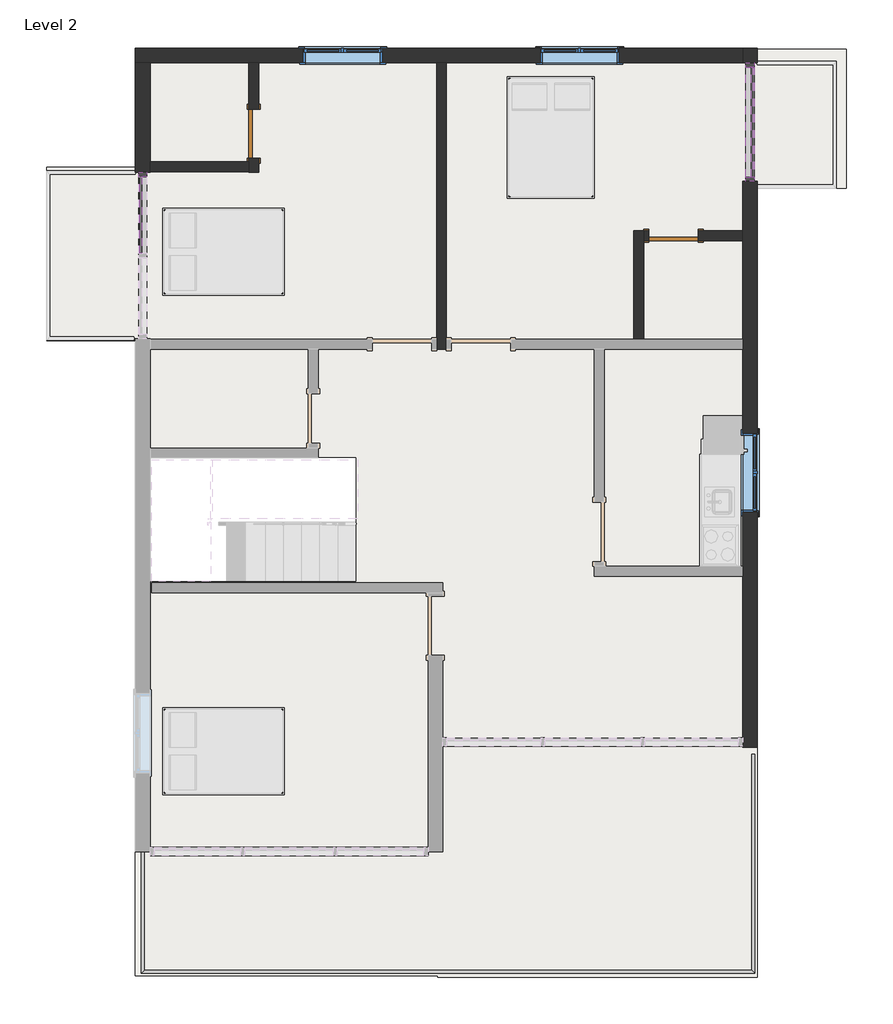
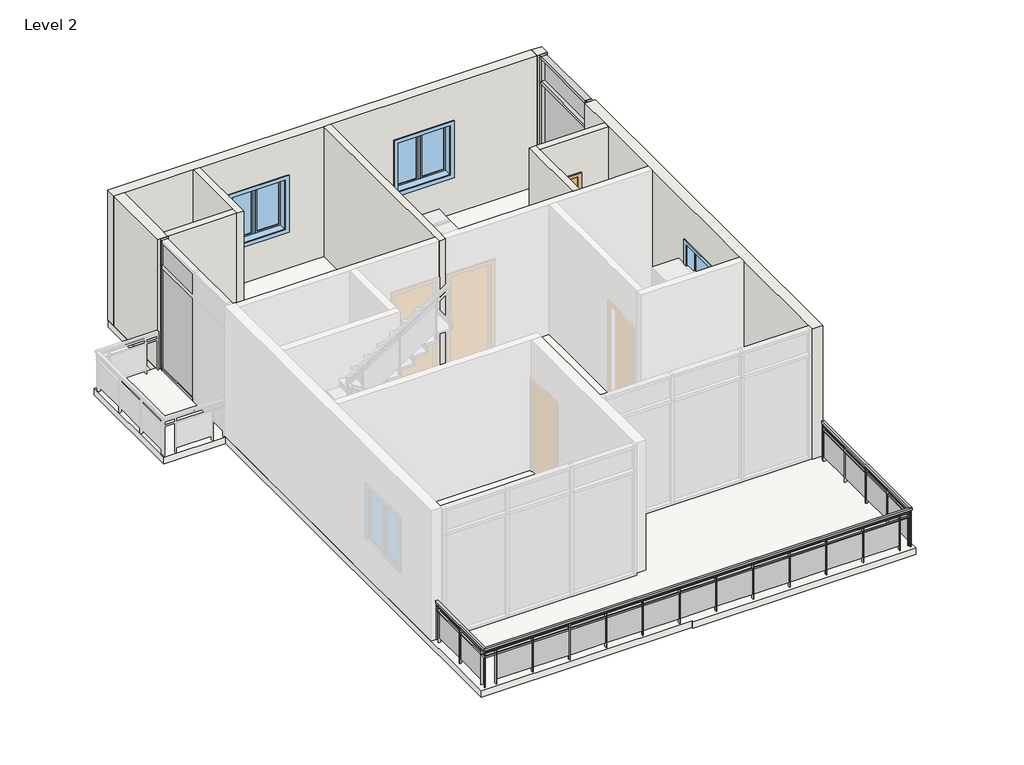
# One storey, part 2 of 3: 10 members, 9 walls, 4 plates, 3 windows, 2 doors, 1 railing, 1 slab.
"""IFC4 building model written with IfcOpenShell, lengths in millimetres."""

from ifc_helpers import new_model, si_unit, frame, origin, place, context, project, spatial, polyline, outline, extrude, faceted_brep, transform, mapped, element, save
from components import single_flush_2_5_e2b13fe9, single_flush_2_5_a9addea7, member_ee409385, member_47bfaf8a, member_43f7a5f1, member_7bc42366, member_cba59155, system_panel_glazed_153bb9bb, system_panel_glazed_f2c52b8f, system_panel_glazed_2d78c1f3, system_panel_glazed_c29578c4, window_8af0dca1

model = new_model("IFC4")

# Units and contexts
model_context = context("Model", 3, world=origin())
ifc_project = project(units=[si_unit("LENGTHUNIT", "METRE", prefix="MILLI")], contexts=[model_context])

# Site, building, storey
site = spatial("IfcSite", under=ifc_project)
building = spatial("IfcBuilding", under=site)
storey = spatial("IfcBuildingStorey", under=building, Name="Level 2", Elevation=3200.4)

# Doors
placement = place(None, origin())
single_flush_2_5_shape = single_flush_2_5_e2b13fe9(model_context)
element("IfcDoor", 1, ObjectType="Single-Flush : 2.5'", at=placement, inside=storey, context=model_context, shape_type="MappedRepresentation", body=[
    mapped(single_flush_2_5_shape, transform((-5884.6647018, 6365.0825188, 3200.4), x_axis=(0.0, -1.0, 0.0), y_axis=(1.0, 0.0, 0.0), z_axis=(0.0, 0.0, 1.0))),
])
single_flush_2_5_2_shape = single_flush_2_5_a9addea7(model_context)
element("IfcDoor", 2, ObjectType="Single-Flush : 2.5'", at=placement, inside=storey, context=model_context, shape_type="MappedRepresentation", body=[
    mapped(single_flush_2_5_2_shape, transform((592.3352982, 4790.2825188, 3200.4), x_axis=(-1.0, 0.0, 0.0), y_axis=(0.0, -1.0, 0.0), z_axis=(0.0, 0.0, 1.0))),
])

# Members
member_shape = member_ee409385(model_context)
element("IfcMember", 3, ObjectType="Rectangular Mullion : 2.5\" x 5\" rectangular", at=placement, inside=storey, context=model_context, shape_type="MappedRepresentation", body=[
    mapped(member_shape, transform((1773.4352982, 5628.4825188, 3200.4), x_axis=(0.0, -1.0, 0.0), y_axis=(-1.0, 0.0, 0.0), z_axis=(0.0, 0.0, -1.0))),
])
element("IfcMember", 4, ObjectType="Rectangular Mullion : 2.5\" x 5\" rectangular", at=placement, inside=storey, context=model_context, shape_type="MappedRepresentation", body=[
    mapped(member_shape, transform((1773.4352982, 7457.2825188, 5638.8), x_axis=(0.0, 1.0, 0.0), y_axis=(-1.0, 0.0, 0.0), z_axis=(0.0, 0.0, 1.0))),
])
member_2_shape = member_47bfaf8a(model_context)
element("IfcMember", 5, ObjectType="Rectangular Mullion : 2.5\" x 5\" rectangular", at=placement, inside=storey, context=model_context, shape_type="MappedRepresentation", body=[
    mapped(member_2_shape, transform((1773.4352982, 5628.4825188, 5638.8), x_axis=(0.0, -1.0, 0.0), y_axis=(-1.0, 0.0, 0.0), z_axis=(0.0, 0.0, -1.0))),
])
element("IfcMember", 6, ObjectType="Rectangular Mullion : 2.5\" x 5\" rectangular", at=placement, inside=storey, context=model_context, shape_type="MappedRepresentation", body=[
    mapped(member_2_shape, transform((1773.4352982, 7457.2825188, 6248.4), x_axis=(0.0, 1.0, 0.0), y_axis=(-1.0, 0.0, 0.0), z_axis=(0.0, 0.0, 1.0))),
])
member_3_shape = member_43f7a5f1(model_context)
element("IfcMember", 7, ObjectType="Rectangular Mullion : 2.5\" x 5\" rectangular", at=placement, inside=storey, context=model_context, shape_type="MappedRepresentation", body=[
    mapped(member_3_shape, transform((-7599.1647018, 5704.6825188, 3200.4), x_axis=(0.0, 0.0, -1.0), y_axis=(-1.0, 0.0, 0.0), z_axis=(0.0, 1.0, 0.0))),
])
element("IfcMember", 8, ObjectType="Rectangular Mullion : 2.5\" x 5\" rectangular", at=placement, inside=storey, context=model_context, shape_type="MappedRepresentation", body=[
    mapped(member_shape, transform((-7599.1647018, 5768.1825188, 5638.8), x_axis=(0.0, 1.0, 0.0), y_axis=(-1.0, 0.0, 0.0), z_axis=(0.0, 0.0, 1.0))),
])
element("IfcMember", 9, ObjectType="Rectangular Mullion : 2.5\" x 5\" rectangular", at=placement, inside=storey, context=model_context, shape_type="MappedRepresentation", body=[
    mapped(member_2_shape, transform((-7599.1647018, 5768.1825188, 6248.4), x_axis=(0.0, 1.0, 0.0), y_axis=(-1.0, 0.0, 0.0), z_axis=(0.0, 0.0, 1.0))),
])
member_4_shape = member_7bc42366(model_context)
element("IfcMember", 10, ObjectType="Rectangular Mullion : 2.5\" x 5\" rectangular", at=placement, inside=storey, context=model_context, shape_type="MappedRepresentation", body=[
    mapped(member_4_shape, transform((1773.4352982, 5691.9825188, 6248.4), x_axis=(0.0, 0.0, 1.0), y_axis=(-1.0, 0.0, 0.0), z_axis=(0.0, -1.0, 0.0))),
])
element("IfcMember", 11, ObjectType="Rectangular Mullion : 2.5\" x 5\" rectangular", at=placement, inside=storey, context=model_context, shape_type="MappedRepresentation", body=[
    mapped(member_4_shape, transform((1773.4352982, 7393.7825188, 3200.4), x_axis=(0.0, 0.0, -1.0), y_axis=(-1.0, 0.0, 0.0), z_axis=(0.0, 1.0, 0.0))),
])
member_5_shape = member_cba59155(model_context)
element("IfcMember", 12, ObjectType="Rectangular Mullion : 2.5\" x 5\" rectangular", at=placement, inside=storey, context=model_context, shape_type="MappedRepresentation", body=[
    mapped(member_5_shape, transform((1773.4352982, 5691.9825188, 5638.8), x_axis=(0.0, 0.0, 1.0), y_axis=(-1.0, 0.0, 0.0), z_axis=(0.0, -1.0, 0.0))),
])

# Plates
system_panel_glazed_shape = system_panel_glazed_153bb9bb(model_context)
element("IfcPlate", 13, ObjectType="System Panel : Glazed", at=placement, inside=storey, context=model_context, shape_type="MappedRepresentation", body=[
    mapped(system_panel_glazed_shape, transform((-7599.1647018, 5110.9575188, 3263.9), x_axis=(0.0, -1.0, 0.0), y_axis=(1.0, 0.0, 0.0), z_axis=(0.0, 0.0, 1.0))),
])
system_panel_glazed_2_shape = system_panel_glazed_f2c52b8f(model_context)
element("IfcPlate", 14, ObjectType="System Panel : Glazed", at=placement, inside=storey, context=model_context, shape_type="MappedRepresentation", body=[
    mapped(system_panel_glazed_2_shape, transform((-7599.1647018, 5110.9575188, 5670.55), x_axis=(0.0, -1.0, 0.0), y_axis=(1.0, 0.0, 0.0), z_axis=(0.0, 0.0, 1.0))),
])
system_panel_glazed_3_shape = system_panel_glazed_2d78c1f3(model_context)
element("IfcPlate", 15, ObjectType="System Panel : Glazed", at=placement, inside=storey, context=model_context, shape_type="MappedRepresentation", body=[
    mapped(system_panel_glazed_3_shape, transform((1773.4352982, 6542.8825188, 3263.9), x_axis=(0.0, -1.0, 0.0), y_axis=(1.0, 0.0, 0.0), z_axis=(0.0, 0.0, 1.0))),
])
system_panel_glazed_4_shape = system_panel_glazed_c29578c4(model_context)
element("IfcPlate", 16, ObjectType="System Panel : Glazed", at=placement, inside=storey, context=model_context, shape_type="MappedRepresentation", body=[
    mapped(system_panel_glazed_4_shape, transform((1773.4352982, 6542.8825188, 5670.55), x_axis=(0.0, -1.0, 0.0), y_axis=(1.0, 0.0, 0.0), z_axis=(0.0, 0.0, 1.0))),
])

# Railing
element("IfcRailing", 17, ObjectType="Glass Panel - Bottom Fill", at=placement, inside=storey, context=model_context, shape_type="SolidModel", body=[
    faceted_brep([(-7573.7647018, -4715.6674812, 4114.8), (-7573.7647018, -4715.6674812, 4064.0), (-7624.5647018, -4715.6674812, 4064.0), (-7624.5647018, -4715.6674812, 4114.8), (-7573.7647018, -6544.4674812, 4114.8), (-7573.7647018, -6544.4674812, 4064.0), (-7624.5647018, -6595.2674812, 4064.0), (-7624.5647018, -6595.2674812, 4114.8), (1798.8352982, -6544.4674812, 4114.8), (1798.8352982, -6544.4674812, 4064.0), (1849.6352982, -6595.2674812, 4064.0), (1849.6352982, -6595.2674812, 4114.8), (1798.8352982, -3217.0674812, 4114.8), (1849.6352982, -3217.0674812, 4114.8), (1849.6352982, -3217.0674812, 4064.0), (1798.8352982, -3217.0674812, 4064.0)], [[[0, 1, 2, 3]], [[1, 0, 4, 5]], [[2, 1, 5, 6]], [[3, 2, 6, 7]], [[0, 3, 7, 4]], [[5, 4, 8, 9]], [[6, 5, 9, 10]], [[7, 6, 10, 11]], [[4, 7, 11, 8]], [[12, 13, 14, 15]], [[9, 8, 12, 15]], [[10, 9, 15, 14]], [[11, 10, 14, 13]], [[8, 11, 13, 12]]]),
    faceted_brep([(-7611.8647018, -4715.6674812, 4025.9), (-7586.4647018, -4715.6674812, 4025.9), (-7586.4647018, -4715.6674812, 4000.5), (-7611.8647018, -4715.6674812, 4000.5), (-7611.8647018, -6582.5674812, 4025.9), (-7586.4647018, -6557.1674812, 4025.9), (-7586.4647018, -6557.1674812, 4000.5), (-7611.8647018, -6582.5674812, 4000.5), (1836.9352982, -6582.5674812, 4025.9), (1811.5352982, -6557.1674812, 4025.9), (1811.5352982, -6557.1674812, 4000.5), (1836.9352982, -6582.5674812, 4000.5), (1836.9352982, -3217.0674812, 4025.9), (1836.9352982, -3217.0674812, 4000.5), (1811.5352982, -3217.0674812, 4000.5), (1811.5352982, -3217.0674812, 4025.9)], [[[0, 1, 2, 3]], [[1, 0, 4, 5]], [[2, 1, 5, 6]], [[3, 2, 6, 7]], [[0, 3, 7, 4]], [[5, 4, 8, 9]], [[6, 5, 9, 10]], [[7, 6, 10, 11]], [[4, 7, 11, 8]], [[12, 13, 14, 15]], [[9, 8, 12, 15]], [[10, 9, 15, 14]], [[11, 10, 14, 13]], [[8, 11, 13, 12]]]),
    faceted_brep([(-7611.8647018, -4715.6674812, 3924.3), (-7586.4647018, -4715.6674812, 3924.3), (-7586.4647018, -4715.6674812, 3898.9), (-7611.8647018, -4715.6674812, 3898.9), (-7611.8647018, -6582.5674812, 3924.3), (-7586.4647018, -6557.1674812, 3924.3), (-7586.4647018, -6557.1674812, 3898.9), (-7611.8647018, -6582.5674812, 3898.9), (1836.9352982, -6582.5674812, 3924.3), (1811.5352982, -6557.1674812, 3924.3), (1811.5352982, -6557.1674812, 3898.9), (1836.9352982, -6582.5674812, 3898.9), (1836.9352982, -3217.0674812, 3924.3), (1836.9352982, -3217.0674812, 3898.9), (1811.5352982, -3217.0674812, 3898.9), (1811.5352982, -3217.0674812, 3924.3)], [[[0, 1, 2, 3]], [[1, 0, 4, 5]], [[2, 1, 5, 6]], [[3, 2, 6, 7]], [[0, 3, 7, 4]], [[5, 4, 8, 9]], [[6, 5, 9, 10]], [[7, 6, 10, 11]], [[4, 7, 11, 8]], [[12, 13, 14, 15]], [[9, 8, 12, 15]], [[10, 9, 15, 14]], [[11, 10, 14, 13]], [[8, 11, 13, 12]]]),
    extrude(outline(polyline([(1849.6352982, -3274.2174812), (1798.8352982, -3274.2174812), (1798.8352982, -3261.5174812), (1849.6352982, -3261.5174812), (1849.6352982, -3274.2174812)])), frame((0.0, 0.0, 3200.4), z_axis=(0.0, 0.0, 1.0), x_axis=(1.0, 0.0, 0.0)), (0.0, 0.0, 1.0), 863.6),
    extrude(outline(polyline([(1817.7001412, -4080.6674812), (1817.7001412, -3267.8674812), (1824.0501412, -3267.8674812), (1824.0501412, -4080.6674812), (1817.7001412, -4080.6674812)])), frame((0.0, 0.0, 3302.0), z_axis=(0.0, 0.0, 1.0), x_axis=(1.0, 0.0, 0.0)), (0.0, 0.0, 1.0), 596.9),
    extrude(outline(polyline([(1849.6352982, -4087.0174812), (1798.8352982, -4087.0174812), (1798.8352982, -4074.3174812), (1849.6352982, -4074.3174812), (1849.6352982, -4087.0174812)])), frame((0.0, 0.0, 3200.4), z_axis=(0.0, 0.0, 1.0), x_axis=(1.0, 0.0, 0.0)), (0.0, 0.0, 1.0), 863.6),
    extrude(outline(polyline([(1817.7001412, -4893.4674812), (1817.7001412, -4080.6674812), (1824.0501412, -4080.6674812), (1824.0501412, -4893.4674812), (1817.7001412, -4893.4674812)])), frame((0.0, 0.0, 3302.0), z_axis=(0.0, 0.0, 1.0), x_axis=(1.0, 0.0, 0.0)), (0.0, 0.0, 1.0), 596.9),
    extrude(outline(polyline([(1849.6352982, -4899.8174812), (1798.8352982, -4899.8174812), (1798.8352982, -4887.1174812), (1849.6352982, -4887.1174812), (1849.6352982, -4899.8174812)])), frame((0.0, 0.0, 3200.4), z_axis=(0.0, 0.0, 1.0), x_axis=(1.0, 0.0, 0.0)), (0.0, 0.0, 1.0), 863.6),
    extrude(outline(polyline([(1817.7001412, -5706.2674812), (1817.7001412, -4893.4674812), (1824.0501412, -4893.4674812), (1824.0501412, -5706.2674812), (1817.7001412, -5706.2674812)])), frame((0.0, 0.0, 3302.0), z_axis=(0.0, 0.0, 1.0), x_axis=(1.0, 0.0, 0.0)), (0.0, 0.0, 1.0), 596.9),
    extrude(outline(polyline([(1849.6352982, -5712.6174812), (1798.8352982, -5712.6174812), (1798.8352982, -5699.9174812), (1849.6352982, -5699.9174812), (1849.6352982, -5712.6174812)])), frame((0.0, 0.0, 3200.4), z_axis=(0.0, 0.0, 1.0), x_axis=(1.0, 0.0, 0.0)), (0.0, 0.0, 1.0), 863.6),
    extrude(outline(polyline([(1817.7001412, -6519.0674812), (1817.7001412, -5706.2674812), (1824.0501412, -5706.2674812), (1824.0501412, -6519.0674812), (1817.7001412, -6519.0674812)])), frame((0.0, 0.0, 3302.0), z_axis=(0.0, 0.0, 1.0), x_axis=(1.0, 0.0, 0.0)), (0.0, 0.0, 1.0), 596.9),
    extrude(outline(polyline([(1849.6352982, -6525.4174812), (1798.8352982, -6525.4174812), (1798.8352982, -6512.7174812), (1849.6352982, -6512.7174812), (1849.6352982, -6525.4174812)])), frame((0.0, 0.0, 3200.4), z_axis=(0.0, 0.0, 1.0), x_axis=(1.0, 0.0, 0.0)), (0.0, 0.0, 1.0), 863.6),
    extrude(outline(polyline([(1576.5852982, -6595.2674812), (1576.5852982, -6544.4674812), (1589.2852982, -6544.4674812), (1589.2852982, -6595.2674812), (1576.5852982, -6595.2674812)])), frame((0.0, 0.0, 3200.4), z_axis=(0.0, 0.0, 1.0), x_axis=(1.0, 0.0, 0.0)), (0.0, 0.0, 1.0), 863.6),
    extrude(outline(polyline([(770.1352982, -6563.3323242), (1582.9352982, -6563.3323242), (1582.9352982, -6569.6823242), (770.1352982, -6569.6823242), (770.1352982, -6563.3323242)])), frame((0.0, 0.0, 3302.0), z_axis=(0.0, 0.0, 1.0), x_axis=(1.0, 0.0, 0.0)), (0.0, 0.0, 1.0), 596.9),
    extrude(outline(polyline([(763.7852982, -6595.2674812), (763.7852982, -6544.4674812), (776.4852982, -6544.4674812), (776.4852982, -6595.2674812), (763.7852982, -6595.2674812)])), frame((0.0, 0.0, 3200.4), z_axis=(0.0, 0.0, 1.0), x_axis=(1.0, 0.0, 0.0)), (0.0, 0.0, 1.0), 863.6),
    extrude(outline(polyline([(-42.6647018, -6563.3323242), (770.1352982, -6563.3323242), (770.1352982, -6569.6823242), (-42.6647018, -6569.6823242), (-42.6647018, -6563.3323242)])), frame((0.0, 0.0, 3302.0), z_axis=(0.0, 0.0, 1.0), x_axis=(1.0, 0.0, 0.0)), (0.0, 0.0, 1.0), 596.9),
    extrude(outline(polyline([(-49.0147018, -6595.2674812), (-49.0147018, -6544.4674812), (-36.3147018, -6544.4674812), (-36.3147018, -6595.2674812), (-49.0147018, -6595.2674812)])), frame((0.0, 0.0, 3200.4), z_axis=(0.0, 0.0, 1.0), x_axis=(1.0, 0.0, 0.0)), (0.0, 0.0, 1.0), 863.6),
    extrude(outline(polyline([(-855.4647018, -6563.3323242), (-42.6647018, -6563.3323242), (-42.6647018, -6569.6823242), (-855.4647018, -6569.6823242), (-855.4647018, -6563.3323242)])), frame((0.0, 0.0, 3302.0), z_axis=(0.0, 0.0, 1.0), x_axis=(1.0, 0.0, 0.0)), (0.0, 0.0, 1.0), 596.9),
    extrude(outline(polyline([(-861.8147018, -6595.2674812), (-861.8147018, -6544.4674812), (-849.1147018, -6544.4674812), (-849.1147018, -6595.2674812), (-861.8147018, -6595.2674812)])), frame((0.0, 0.0, 3200.4), z_axis=(0.0, 0.0, 1.0), x_axis=(1.0, 0.0, 0.0)), (0.0, 0.0, 1.0), 863.6),
    extrude(outline(polyline([(-1668.2647018, -6563.3323242), (-855.4647018, -6563.3323242), (-855.4647018, -6569.6823242), (-1668.2647018, -6569.6823242), (-1668.2647018, -6563.3323242)])), frame((0.0, 0.0, 3302.0), z_axis=(0.0, 0.0, 1.0), x_axis=(1.0, 0.0, 0.0)), (0.0, 0.0, 1.0), 596.9),
    extrude(outline(polyline([(-1674.6147018, -6595.2674812), (-1674.6147018, -6544.4674812), (-1661.9147018, -6544.4674812), (-1661.9147018, -6595.2674812), (-1674.6147018, -6595.2674812)])), frame((0.0, 0.0, 3200.4), z_axis=(0.0, 0.0, 1.0), x_axis=(1.0, 0.0, 0.0)), (0.0, 0.0, 1.0), 863.6),
    extrude(outline(polyline([(-2481.0647018, -6563.3323242), (-1668.2647018, -6563.3323242), (-1668.2647018, -6569.6823242), (-2481.0647018, -6569.6823242), (-2481.0647018, -6563.3323242)])), frame((0.0, 0.0, 3302.0), z_axis=(0.0, 0.0, 1.0), x_axis=(1.0, 0.0, 0.0)), (0.0, 0.0, 1.0), 596.9),
    extrude(outline(polyline([(-2487.4147018, -6595.2674812), (-2487.4147018, -6544.4674812), (-2474.7147018, -6544.4674812), (-2474.7147018, -6595.2674812), (-2487.4147018, -6595.2674812)])), frame((0.0, 0.0, 3200.4), z_axis=(0.0, 0.0, 1.0), x_axis=(1.0, 0.0, 0.0)), (0.0, 0.0, 1.0), 863.6),
    extrude(outline(polyline([(-3293.8647018, -6563.3323242), (-2481.0647018, -6563.3323242), (-2481.0647018, -6569.6823242), (-3293.8647018, -6569.6823242), (-3293.8647018, -6563.3323242)])), frame((0.0, 0.0, 3302.0), z_axis=(0.0, 0.0, 1.0), x_axis=(1.0, 0.0, 0.0)), (0.0, 0.0, 1.0), 596.9),
    extrude(outline(polyline([(-3300.2147018, -6595.2674812), (-3300.2147018, -6544.4674812), (-3287.5147018, -6544.4674812), (-3287.5147018, -6595.2674812), (-3300.2147018, -6595.2674812)])), frame((0.0, 0.0, 3200.4), z_axis=(0.0, 0.0, 1.0), x_axis=(1.0, 0.0, 0.0)), (0.0, 0.0, 1.0), 863.6),
    extrude(outline(polyline([(-4106.6647018, -6563.3323242), (-3293.8647018, -6563.3323242), (-3293.8647018, -6569.6823242), (-4106.6647018, -6569.6823242), (-4106.6647018, -6563.3323242)])), frame((0.0, 0.0, 3302.0), z_axis=(0.0, 0.0, 1.0), x_axis=(1.0, 0.0, 0.0)), (0.0, 0.0, 1.0), 596.9),
    extrude(outline(polyline([(-4113.0147018, -6595.2674812), (-4113.0147018, -6544.4674812), (-4100.3147018, -6544.4674812), (-4100.3147018, -6595.2674812), (-4113.0147018, -6595.2674812)])), frame((0.0, 0.0, 3200.4), z_axis=(0.0, 0.0, 1.0), x_axis=(1.0, 0.0, 0.0)), (0.0, 0.0, 1.0), 863.6),
    extrude(outline(polyline([(-4919.4647018, -6563.3323242), (-4106.6647018, -6563.3323242), (-4106.6647018, -6569.6823242), (-4919.4647018, -6569.6823242), (-4919.4647018, -6563.3323242)])), frame((0.0, 0.0, 3302.0), z_axis=(0.0, 0.0, 1.0), x_axis=(1.0, 0.0, 0.0)), (0.0, 0.0, 1.0), 596.9),
    extrude(outline(polyline([(-4925.8147018, -6595.2674812), (-4925.8147018, -6544.4674812), (-4913.1147018, -6544.4674812), (-4913.1147018, -6595.2674812), (-4925.8147018, -6595.2674812)])), frame((0.0, 0.0, 3200.4), z_axis=(0.0, 0.0, 1.0), x_axis=(1.0, 0.0, 0.0)), (0.0, 0.0, 1.0), 863.6),
    extrude(outline(polyline([(-5732.2647018, -6563.3323242), (-4919.4647018, -6563.3323242), (-4919.4647018, -6569.6823242), (-5732.2647018, -6569.6823242), (-5732.2647018, -6563.3323242)])), frame((0.0, 0.0, 3302.0), z_axis=(0.0, 0.0, 1.0), x_axis=(1.0, 0.0, 0.0)), (0.0, 0.0, 1.0), 596.9),
    extrude(outline(polyline([(-5738.6147018, -6595.2674812), (-5738.6147018, -6544.4674812), (-5725.9147018, -6544.4674812), (-5725.9147018, -6595.2674812), (-5738.6147018, -6595.2674812)])), frame((0.0, 0.0, 3200.4), z_axis=(0.0, 0.0, 1.0), x_axis=(1.0, 0.0, 0.0)), (0.0, 0.0, 1.0), 863.6),
    extrude(outline(polyline([(-6545.0647018, -6563.3323242), (-5732.2647018, -6563.3323242), (-5732.2647018, -6569.6823242), (-6545.0647018, -6569.6823242), (-6545.0647018, -6563.3323242)])), frame((0.0, 0.0, 3302.0), z_axis=(0.0, 0.0, 1.0), x_axis=(1.0, 0.0, 0.0)), (0.0, 0.0, 1.0), 596.9),
    extrude(outline(polyline([(-6551.4147018, -6595.2674812), (-6551.4147018, -6544.4674812), (-6538.7147018, -6544.4674812), (-6538.7147018, -6595.2674812), (-6551.4147018, -6595.2674812)])), frame((0.0, 0.0, 3200.4), z_axis=(0.0, 0.0, 1.0), x_axis=(1.0, 0.0, 0.0)), (0.0, 0.0, 1.0), 863.6),
    extrude(outline(polyline([(-7357.8647018, -6563.3323242), (-6545.0647018, -6563.3323242), (-6545.0647018, -6569.6823242), (-7357.8647018, -6569.6823242), (-7357.8647018, -6563.3323242)])), frame((0.0, 0.0, 3302.0), z_axis=(0.0, 0.0, 1.0), x_axis=(1.0, 0.0, 0.0)), (0.0, 0.0, 1.0), 596.9),
    extrude(outline(polyline([(-7364.2147018, -6595.2674812), (-7364.2147018, -6544.4674812), (-7351.5147018, -6544.4674812), (-7351.5147018, -6595.2674812), (-7364.2147018, -6595.2674812)])), frame((0.0, 0.0, 3200.4), z_axis=(0.0, 0.0, 1.0), x_axis=(1.0, 0.0, 0.0)), (0.0, 0.0, 1.0), 863.6),
    extrude(outline(polyline([(-7624.5647018, -6449.2174812), (-7573.7647018, -6449.2174812), (-7573.7647018, -6461.9174812), (-7624.5647018, -6461.9174812), (-7624.5647018, -6449.2174812)])), frame((0.0, 0.0, 3200.4), z_axis=(0.0, 0.0, 1.0), x_axis=(1.0, 0.0, 0.0)), (0.0, 0.0, 1.0), 863.6),
    extrude(outline(polyline([(-7592.6295448, -5642.7674812), (-7592.6295448, -6455.5674812), (-7598.9795448, -6455.5674812), (-7598.9795448, -5642.7674812), (-7592.6295448, -5642.7674812)])), frame((0.0, 0.0, 3302.0), z_axis=(0.0, 0.0, 1.0), x_axis=(1.0, 0.0, 0.0)), (0.0, 0.0, 1.0), 596.9),
    extrude(outline(polyline([(-7624.5647018, -5636.4174812), (-7573.7647018, -5636.4174812), (-7573.7647018, -5649.1174812), (-7624.5647018, -5649.1174812), (-7624.5647018, -5636.4174812)])), frame((0.0, 0.0, 3200.4), z_axis=(0.0, 0.0, 1.0), x_axis=(1.0, 0.0, 0.0)), (0.0, 0.0, 1.0), 863.6),
    extrude(outline(polyline([(-7592.6295448, -4829.9674812), (-7592.6295448, -5642.7674812), (-7598.9795448, -5642.7674812), (-7598.9795448, -4829.9674812), (-7592.6295448, -4829.9674812)])), frame((0.0, 0.0, 3302.0), z_axis=(0.0, 0.0, 1.0), x_axis=(1.0, 0.0, 0.0)), (0.0, 0.0, 1.0), 596.9),
    extrude(outline(polyline([(-7624.5647018, -4823.6174812), (-7573.7647018, -4823.6174812), (-7573.7647018, -4836.3174812), (-7624.5647018, -4836.3174812), (-7624.5647018, -4823.6174812)])), frame((0.0, 0.0, 3200.4), z_axis=(0.0, 0.0, 1.0), x_axis=(1.0, 0.0, 0.0)), (0.0, 0.0, 1.0), 863.6),
    extrude(outline(polyline([(1814.7102982, -6579.3924812), (1814.7102982, -6560.3424812), (1833.7602982, -6560.3424812), (1833.7602982, -6579.3924812), (1814.7102982, -6579.3924812)])), frame((0.0, 0.0, 3200.4), z_axis=(0.0, 0.0, 1.0), x_axis=(1.0, 0.0, 0.0)), (0.0, 0.0, 1.0), 863.6),
    extrude(outline(polyline([(-7608.6897018, -6560.3424812), (-7589.6397018, -6560.3424812), (-7589.6397018, -6579.3924812), (-7608.6897018, -6579.3924812), (-7608.6897018, -6560.3424812)])), frame((0.0, 0.0, 3200.4), z_axis=(0.0, 0.0, 1.0), x_axis=(1.0, 0.0, 0.0)), (0.0, 0.0, 1.0), 863.6),
    extrude(outline(polyline([(1833.7602982, -3229.7674812), (1814.7102982, -3229.7674812), (1814.7102982, -3210.7174812), (1833.7602982, -3210.7174812), (1833.7602982, -3229.7674812)])), frame((0.0, 0.0, 3200.4), z_axis=(0.0, 0.0, 1.0), x_axis=(1.0, 0.0, 0.0)), (0.0, 0.0, 1.0), 863.6),
    extrude(outline(polyline([(-7608.6897018, -4709.3174812), (-7589.6397018, -4709.3174812), (-7589.6397018, -4728.3674812), (-7608.6897018, -4728.3674812), (-7608.6897018, -4709.3174812)])), frame((0.0, 0.0, 3200.4), z_axis=(0.0, 0.0, 1.0), x_axis=(1.0, 0.0, 0.0)), (0.0, 0.0, 1.0), 863.6),
])

# Slab
element("IfcSlab", 18, ObjectType="6\"", at=placement, inside=storey, context=model_context, shape_type="SweptSolid", body=[
    extrude(outline(polyline([(-7713.4647018, 7666.8325188), (3259.3352982, 7666.8325188), (3259.3352982, 5526.8825188), (1887.7352982, 5526.8825188), (1887.7352982, -6658.7674812), (-3043.7591614, -6658.7674812), (-3043.7591614, -6633.3674812), (-7713.4647018, -6633.3674812), (-7713.4647018, 3171.0325188), (-9085.0647018, 3171.0325188), (-9085.0647018, 5844.3825188), (-7713.4647018, 5844.3825188), (-7713.4647018, 7666.8325188)]), holes=[polyline([(-4313.7591614, 1361.2825188), (-7548.3647018, 1361.2825188), (-7548.3647018, -543.1950563), (-4313.7591614, -543.1950563), (-4313.7591614, 1361.2825188)])]), frame((0.0, 0.0, 3048.0), z_axis=(0.0, 0.0, 1.0), x_axis=(1.0, 0.0, 0.0)), (0.0, 0.0, 1.0), 152.4),
])

# Walls
element("IfcWall", 19, ObjectType="6\"", at=placement, inside=storey, context=model_context, shape_type="Brep", body=[
    faceted_brep([(-3065.2647018, 7457.2825188, 3200.4), (-3065.2647018, 3190.0825188, 3200.4), (-3065.2647018, 3037.6825188, 3200.4), (-3065.2647018, 3037.6825188, 6248.4), (-3065.2647018, 3190.0825188, 6248.4), (-3065.2647018, 7457.2825188, 6248.4), (-2912.8647018, 7457.2825188, 3200.4), (-2912.8647018, 7457.2825188, 6248.4), (-2912.8647018, 3190.0825188, 6248.4), (-2912.8647018, 3037.6825188, 6248.4), (-2912.8647018, 3037.6825188, 3200.4), (-2912.8647018, 3190.0825188, 3200.4)], [[[0, 1, 2, 3, 4, 5]], [[6, 7, 8, 9, 10, 11]], [[2, 1, 0, 6, 11, 10]], [[5, 4, 3, 9, 8, 7]], [[0, 5, 7, 6]], [[3, 2, 10, 9]]]),
])
element("IfcWall", 20, ObjectType="6\"", at=placement, inside=storey, context=model_context, shape_type="SweptSolid", body=[
    extrude(outline(polyline([(-7484.8647018, 5933.2825188), (-5960.8647018, 5933.2825188), (-5960.8647018, 5780.8825188), (-7484.8647018, 5780.8825188), (-7484.8647018, 5933.2825188)])), frame((0.0, 0.0, 3200.4), z_axis=(0.0, 0.0, 1.0), x_axis=(1.0, 0.0, 0.0)), (0.0, 0.0, 1.0), 3048.0),
])
element("IfcWall", 21, ObjectType="6\"", at=placement, inside=storey, context=model_context, shape_type="Brep", body=[
    faceted_brep([(135.1352982, 3190.0825188, 3200.4), (135.1352982, 4714.0825188, 3200.4), (135.1352982, 4866.4825188, 3200.4), (135.1352982, 4866.4825188, 6248.4), (135.1352982, 4714.0825188, 6248.4), (135.1352982, 3190.0825188, 6248.4), (-17.2647018, 3190.0825188, 3200.4), (-17.2647018, 3190.0825188, 6248.4), (-17.2647018, 4866.4825188, 6248.4), (-17.2647018, 4866.4825188, 3200.4)], [[[0, 1, 2, 3, 4, 5]], [[6, 7, 8, 9]], [[2, 1, 0, 6, 9]], [[5, 4, 3, 8, 7]], [[0, 5, 7, 6]], [[3, 2, 9, 8]]]),
])
element("IfcWall", 22, ObjectType="6\"", at=placement, inside=storey, context=model_context, shape_type="SweptSolid", body=[
    extrude(outline(polyline([(3200.4, 135.1352982), (3200.4, 211.3352982), (5334.0, 211.3352982), (5334.0, 973.3352982), (3200.4, 973.3352982), (3200.4, 1659.1352982), (6248.4, 1659.1352982), (6248.4, 135.1352982), (3200.4, 135.1352982)])), frame((0.0, 4714.0825188, 0.0), z_axis=(0.0, 1.0, 0.0), x_axis=(0.0, 0.0, 1.0)), (0.0, 0.0, 1.0), 152.4),
])
element("IfcWall", 23, ObjectType="6\"", at=placement, inside=storey, context=model_context, shape_type="Brep", body=[
    faceted_brep([(-5808.4647018, 5774.5325188, 3200.4), (-5808.4647018, 5984.0825188, 3200.4), (-5808.4647018, 5984.0825188, 5334.0), (-5808.4647018, 6746.0825188, 5334.0), (-5808.4647018, 6746.0825188, 3200.4), (-5808.4647018, 7457.2825188, 3200.4), (-5808.4647018, 7457.2825188, 6248.4), (-5808.4647018, 5774.5325188, 6248.4), (-5960.8647018, 5984.0825188, 5334.0), (-5960.8647018, 5984.0825188, 3200.4), (-5960.8647018, 5933.2825188, 3200.4), (-5960.8647018, 5780.8825188, 3200.4), (-5960.8647018, 5774.5325188, 3200.4), (-5960.8647018, 5774.5325188, 6248.4), (-5960.8647018, 5780.8825188, 6248.4), (-5960.8647018, 5933.2825188, 6248.4), (-5960.8647018, 7457.2825188, 6248.4), (-5960.8647018, 7457.2825188, 3200.4), (-5960.8647018, 6746.0825188, 3200.4), (-5960.8647018, 6746.0825188, 5334.0)], [[[0, 1, 2, 3, 4, 5, 6, 7]], [[8, 9, 10, 11, 12, 13, 14, 15, 16, 17, 18, 19]], [[18, 17, 5, 4]], [[12, 11, 10, 9, 1, 0]], [[7, 6, 16, 15, 14, 13]], [[0, 7, 13, 12]], [[6, 5, 17, 16]], [[2, 1, 9, 8]], [[3, 2, 8, 19]], [[4, 3, 19, 18]]]),
])
element("IfcWall", 24, ObjectType="9\"", at=placement, inside=storey, context=model_context, shape_type="Brep", body=[
    faceted_brep([(-7713.4647018, 7457.2825188, 3200.4), (-7713.4647018, 5768.1825188, 3200.4), (-7713.4647018, 5768.1825188, 6248.4), (-7713.4647018, 7457.2825188, 6248.4), (-7484.8647018, 7457.2825188, 3200.4), (-7484.8647018, 7457.2825188, 6248.4), (-7484.8647018, 5933.2825188, 6248.4), (-7484.8647018, 5780.8825188, 6248.4), (-7484.8647018, 5768.1825188, 6248.4), (-7484.8647018, 5768.1825188, 3200.4), (-7484.8647018, 5780.8825188, 3200.4), (-7484.8647018, 5933.2825188, 3200.4)], [[[0, 1, 2, 3]], [[4, 5, 6, 7, 8, 9, 10, 11]], [[1, 0, 4, 11, 10, 9]], [[2, 1, 9, 8]], [[3, 2, 8, 7, 6, 5]], [[0, 3, 5, 4]]]),
])
element("IfcWall", 25, ObjectType="9\"", at=placement, inside=storey, context=model_context, shape_type="Brep", body=[
    faceted_brep([(1887.7352982, -3102.2450563, 3200.4), (1887.7352982, 5628.4825188, 3200.4), (1887.7352982, 5628.4825188, 6248.4), (1887.7352982, -3102.2450563, 6248.4), (1887.7352982, 523.0825188, 5334.0), (1887.7352982, 1742.2825188, 5334.0), (1887.7352982, 1742.2825188, 4114.8), (1887.7352982, 523.0825188, 4114.8), (1659.1352982, -3102.2450563, 3200.4), (1659.1352982, -3102.2450563, 6248.4), (1659.1352982, -467.5174812, 6248.4), (1659.1352982, -315.1174812, 6248.4), (1659.1352982, 3037.6825188, 6248.4), (1659.1352982, 3190.0825188, 6248.4), (1659.1352982, 4714.0825188, 6248.4), (1659.1352982, 4866.4825188, 6248.4), (1659.1352982, 5628.4825188, 6248.4), (1659.1352982, 5628.4825188, 3200.4), (1659.1352982, 4866.4825188, 3200.4), (1659.1352982, 4714.0825188, 3200.4), (1659.1352982, 3190.0825188, 3200.4), (1659.1352982, 3037.6825188, 3200.4), (1659.1352982, -315.1174812, 3200.4), (1659.1352982, -467.5174812, 3200.4), (1659.1352982, 523.0825188, 5334.0), (1659.1352982, 523.0825188, 4114.8), (1659.1352982, 1742.2825188, 4114.8), (1659.1352982, 1742.2825188, 5334.0)], [[[0, 1, 2, 3], [4, 5, 6, 7]], [[8, 9, 10, 11, 12, 13, 14, 15, 16, 17, 18, 19, 20, 21, 22, 23], [24, 25, 26, 27]], [[1, 0, 8, 23, 22, 21, 20, 19, 18, 17]], [[2, 1, 17, 16]], [[3, 2, 16, 15, 14, 13, 12, 11, 10, 9]], [[0, 3, 9, 8]], [[25, 24, 4, 7]], [[26, 25, 7, 6]], [[27, 26, 6, 5]], [[24, 27, 5, 4]]]),
])
element("IfcWall", 26, ObjectType="9\"", at=placement, inside=storey, context=model_context, shape_type="Brep", body=[
    faceted_brep([(-7713.4647018, 7457.2825188, 3200.4), (-7484.8647018, 7457.2825188, 3200.4), (-5960.8647018, 7457.2825188, 3200.4), (-5808.4647018, 7457.2825188, 3200.4), (-3065.2647018, 7457.2825188, 3200.4), (-2912.8647018, 7457.2825188, 3200.4), (1659.1352982, 7457.2825188, 3200.4), (1659.1352982, 7457.2825188, 6248.4), (-2912.8647018, 7457.2825188, 6248.4), (-3065.2647018, 7457.2825188, 6248.4), (-5808.4647018, 7457.2825188, 6248.4), (-5960.8647018, 7457.2825188, 6248.4), (-7484.8647018, 7457.2825188, 6248.4), (-7713.4647018, 7457.2825188, 6248.4), (-3903.4647018, 7457.2825188, 5334.0), (-3903.4647018, 7457.2825188, 4114.8), (-5122.6647018, 7457.2825188, 4114.8), (-5122.6647018, 7457.2825188, 5334.0), (-245.8647018, 7457.2825188, 5334.0), (-245.8647018, 7457.2825188, 4114.8), (-1465.0647018, 7457.2825188, 4114.8), (-1465.0647018, 7457.2825188, 5334.0), (-7713.4647018, 7685.8825188, 3200.4), (-7713.4647018, 7685.8825188, 6248.4), (1659.1352982, 7685.8825188, 6248.4), (1659.1352982, 7685.8825188, 3200.4), (-3903.4647018, 7685.8825188, 5334.0), (-5122.6647018, 7685.8825188, 5334.0), (-5122.6647018, 7685.8825188, 4114.8), (-3903.4647018, 7685.8825188, 4114.8), (-245.8647018, 7685.8825188, 5334.0), (-1465.0647018, 7685.8825188, 5334.0), (-1465.0647018, 7685.8825188, 4114.8), (-245.8647018, 7685.8825188, 4114.8)], [[[0, 1, 2, 3, 4, 5, 6, 7, 8, 9, 10, 11, 12, 13], [14, 15, 16, 17], [18, 19, 20, 21]], [[22, 23, 24, 25], [26, 27, 28, 29], [30, 31, 32, 33]], [[6, 5, 4, 3, 2, 1, 0, 22, 25]], [[13, 12, 11, 10, 9, 8, 7, 24, 23]], [[7, 6, 25, 24]], [[0, 13, 23, 22]], [[15, 14, 26, 29]], [[16, 15, 29, 28]], [[17, 16, 28, 27]], [[14, 17, 27, 26]], [[19, 18, 30, 33]], [[20, 19, 33, 32]], [[21, 20, 32, 31]], [[18, 21, 31, 30]]]),
])
element("IfcWall", 27, ObjectType="9\"", at=placement, inside=storey, context=model_context, shape_type="SweptSolid", body=[
    extrude(outline(polyline([(1887.7352982, 7685.8825188), (1887.7352982, 7457.2825188), (1659.1352982, 7457.2825188), (1659.1352982, 7685.8825188), (1887.7352982, 7685.8825188)])), frame((0.0, 0.0, 3200.4), z_axis=(0.0, 0.0, 1.0), x_axis=(1.0, 0.0, 0.0)), (0.0, 0.0, 1.0), 3048.0),
])

# Windows
window_shape = window_8af0dca1(model_context)
element("IfcWindow", 28, ObjectType="Casement Dbl with Trim : 48\" x 48\"", at=placement, inside=storey, context=model_context, shape_type="MappedRepresentation", body=[
    mapped(window_shape, transform((-4513.0647018, 7552.5325188, 3352.8), x_axis=(1.0, 0.0, 0.0), y_axis=(0.0, 1.0, 0.0), z_axis=(0.0, 0.0, 1.0))),
])
element("IfcWindow", 29, ObjectType="Casement Dbl with Trim : 48\" x 48\"", at=placement, inside=storey, context=model_context, shape_type="MappedRepresentation", body=[
    mapped(window_shape, transform((-855.4647018, 7552.5325188, 3352.8), x_axis=(1.0, 0.0, 0.0), y_axis=(0.0, 1.0, 0.0), z_axis=(0.0, 0.0, 1.0))),
])
element("IfcWindow", 30, ObjectType="Casement Dbl with Trim : 48\" x 48\"", at=placement, inside=storey, context=model_context, shape_type="MappedRepresentation", body=[
    mapped(window_shape, transform((1754.3852982, 1132.6825188, 3352.8), x_axis=(0.0, -1.0, 0.0), y_axis=(1.0, 0.0, 0.0), z_axis=(0.0, 0.0, 1.0))),
])

save(model, "model.ifc")

# Revit data of these elements
# Type "Single-Flush : 2.5'"
#   Type Mark = "8"
#   Construction Type Id = "MDOOR"
#   Assembly Code = "C1020"
#   Analytic Construction = "Metal"
#   Thickness = 0' - 2"
#   Heat Transfer Coefficient (U) = 0.651978 BTU/(h·ft²·°F)
#   Height = 7' - 0"
#   Trim Projection Ext = 0' - 1"
#   Trim Projection Int = 0' - 1"
#   Trim Width = 0' - 3"
#   Width = 2' - 6"
#   Define Thermal Properties by = 1
#   Door Material = Door - Panel
#   Frame Material = Door - Frame
#   Visual Light Transmittance = 0
#   Solar Heat Gain Coefficient = 0
#   Function = (empty or 0)
#   Wall Closure = (empty or 0)
# Type "Rectangular Mullion : 2.5\" x 5\" rectangular"
#   built-in parameter 1007304 = 0.416667 (stored number, unit not read)
#   built-in parameter 1007301 = 0.104167 (stored number, unit not read)
#   built-in parameter 1007300 = 0.104167 (stored number, unit not read)
# Type "System Panel : Glazed"
#   Construction Type Id = "GSP4R"
#   Analytic Construction = "1/8 in Pilkington single glazing"
#   Visual Light Transmittance = 0.9
#   Solar Heat Gain Coefficient = 0.86
#   Heat Transfer Coefficient (U) = 1.18115 BTU/(h·ft²·°F)
# Type "Glass Panel - Bottom Fill"
#   Assembly Code = "C2010400"
#   built-in parameter 1008612 = 0.0416667 (stored number, unit not read)
#   built-in parameter 1008611 = 0.0416667 (stored number, unit not read)
#   built-in parameter 1008609 = 0.333333 (stored number, unit not read)
#   built-in parameter 1008604 = 0.166667 (stored number, unit not read)
#   built-in parameter 1008603 = 0.166667 (stored number, unit not read)
#   Railing Height = 3' - 0"
#   built-in parameter 1008630 = 2
#   built-in parameter 1008610 = 2
#   built-in parameter 1008618 = Baluster - Square : 3/4"
# Type "6\""
#   Assembly Code = "B1010"
#   Function = 0
#   Layers, outside or top first: 0' - 6" "floor" (function 1)
# Type "6\""
#   Assembly Code = "B2010"
#   Layers, outside or top first: 0' - 6" "inner wall" (function 1)
# Type "9\""
#   Assembly Code = "B2010"
#   Layers, outside or top first: 0' - 9" "ext wall" (function 1)
# Type "Casement Dbl with Trim : 48\" x 48\""
#   Type Mark = "10"
#   Construction Type Id = "GSP4R"
#   Assembly Code = "B2020100"
#   Analytic Construction = "1/8 in Pilkington single glazing"
#   Visual Light Transmittance = 0.9
#   Solar Heat Gain Coefficient = 0.78
#   Heat Transfer Coefficient (U) = 0.6496 BTU/(h·ft²·°F)
#   Height = 4' - 0"
#   Default Sill Height = 2' - 6"
#   Trim Projection - Ext. = 0' - 0 1/2"
#   Trim Projection - Int. = 0' - 0 3/4"
#   Trim Width - Exterior = 0' - 3 1/2"
#   Trim Width - Interior = 0' - 3 1/2"
#   Width = 4' - 0"
#   Window Inset = 0' - 0 3/4"
#   Define Thermal Properties by = 1
#   Glass Pane Material = Glass
#   Sash Material = Sash
#   Trim Exterior Material = Trim
#   Trim Interior Material = Trim
#   Wall Closure = (empty or 0)
# Elements 1, 2 (IfcDoor, "Single-Flush : 2.5'")
#   Phase Created = New Construction
#   Materials on its faces: "Door - Frame", "Door - Panel"
# Elements 3, 4, 5, 6, 7, 8, 9, 10, 11, 12 (IfcMember, "Rectangular Mullion : 2.5\" x 5\" rectangular")
#   Phase Created = New Construction
#   Materials on its faces: "Aluminum"
# Elements 13, 14, 15, 16 (IfcPlate, "System Panel : Glazed")
#   Phase Created = New Construction
#   Materials on its faces: "Glass"
# Element 17 (IfcRailing, "Glass Panel - Bottom Fill")
#   Phase Created = New Construction
#   Materials on its faces: "Glass"
# Element 18 (IfcSlab, "6\"")
#   Height Offset From Level = 0' - 0"
#   Phase Created = New Construction
#   Materials on its faces: "floor"
# Elements 19, 20, 21, 22, 23 (IfcWall, "6\"")
#   Top Offset = 0' - 0"
#   Base Offset = 0' - 0"
#   Unconnected Height = 10' - 0"
#   wall height = 10' - 0"
#   Phase Created = New Construction
#   Base Constraint = Level 2
#   Materials on its faces: "inner wall"
# Elements 24, 25, 26 (IfcWall, "9\"")
#   Top Offset = 0' - 0"
#   Base Offset = 0' - 0"
#   Unconnected Height = 10' - 0"
#   wall height = 10' - 0"
#   Phase Created = New Construction
#   Base Constraint = Level 2
#   Materials on its faces: "ext wall", "inner wall"
# Element 27 (IfcWall, "9\"")
#   Top Offset = 0' - 0"
#   Base Offset = 0' - 0"
#   Unconnected Height = 10' - 0"
#   wall height = 10' - 0"
#   Phase Created = New Construction
#   Base Constraint = Level 2
#   Materials on its faces: "ext wall"
# Element 28 (IfcWindow, "Casement Dbl with Trim : 48\" x 48\"")
#   Mark = "10"
#   Phase Created = New Construction
#   Materials on its faces: "Sash", "Trim", "Glass"
# Element 29 (IfcWindow, "Casement Dbl with Trim : 48\" x 48\"")
#   Mark = "11"
#   Phase Created = New Construction
#   Materials on its faces: "Sash", "Trim", "Glass"
# Element 30 (IfcWindow, "Casement Dbl with Trim : 48\" x 48\"")
#   Mark = "12"
#   Phase Created = New Construction
#   Materials on its faces: "Sash", "Trim", "Glass"
# Materials
#   "Door - Panel": class "Wood", colour RGB 210 159 95, transparency 0
#   "Door - Frame": colour RGB 118 70 51, transparency 0
#   "floor": class "Generic", colour RGB 128 100 74, transparency 0, Cost = 0
#   "inner wall": class "Generic", colour RGB 230 213 172, transparency 0, Cost = 0
#   "ext wall": class "Generic", colour RGB 153 153 153, transparency 0, Cost = 0
#   "Glass": class "Glass", colour RGB 0 128 192, transparency 0.75, Description = "Soda Lime Glass", Cost = 0
#   "Sash": class "Wood", colour RGB 224 178 126, transparency 0
#   "Trim": class "Wood", colour RGB 224 178 126, transparency 0
#   "Aluminum": class "Metal", colour RGB 247 247 247, transparency 0, Description = "Aluminum 6061", Cost = 0
